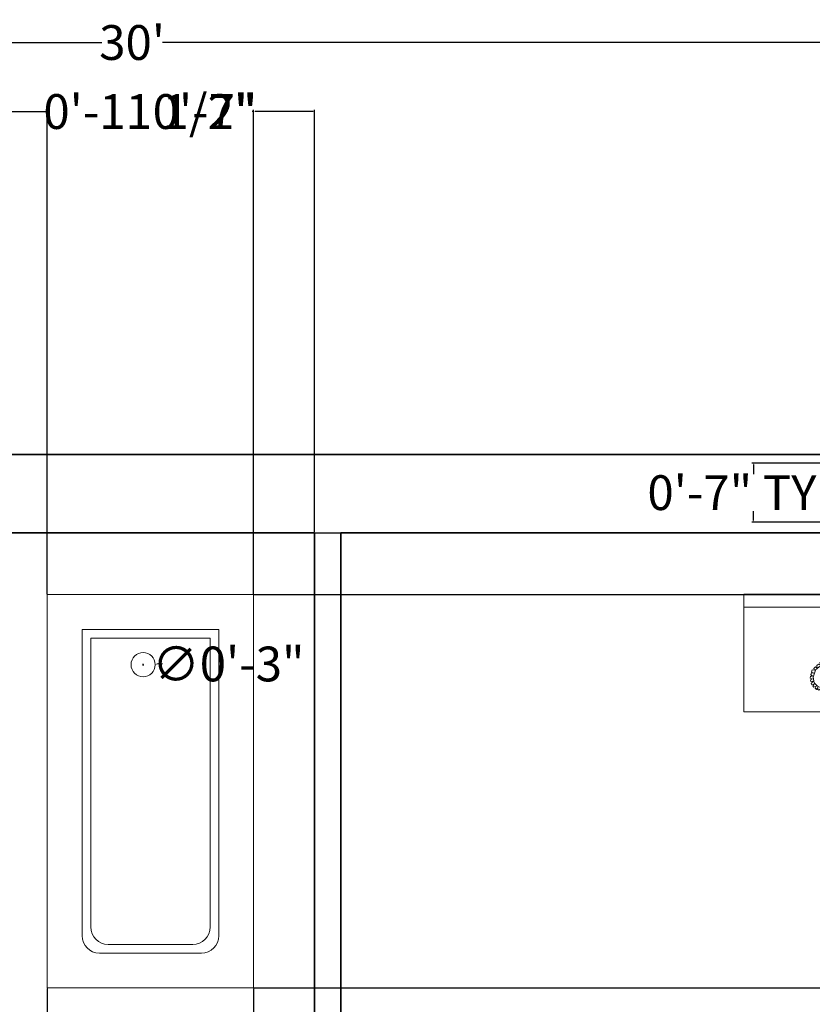
# Model space of a CAD drawing. Units: inches. Extents: x 311 to 754, y 60 to 497.
# Tile 10 of 11: x 530 to 621, y 384 to 497. Entities that reach past the tile are written whole.
import ezdxf

# ---------------------------------------------------------------- set-up
doc = ezdxf.new("R2010")
doc.units = ezdxf.units.IN
doc.header["$MEASUREMENT"] = 0
for name, color, linetype, lineweight in [('A-ANNO-DIMS', 2, 'Continuous', 18), ('A-FLOR-FIXT', 9, 'Continuous', 18), ('A-WALL', 7, 'Continuous', 35), ('beds', 70, 'Continuous', 13)]:
    doc.layers.add(name, color=color, linetype=linetype, lineweight=lineweight)
doc.styles.get("Standard").update_dxf_attribs({"font": 'arial.ttf'})
doc.dimstyles.get("Standard").update_dxf_attribs({"dimtxt": 4, "dimasz": 0.18, "dimexe": 0.18, "dimexo": 0.0625, "dimgap": 0.09, "dimtad": 0, "dimtih": 1, "dimtoh": 1, "dimdec": 0, "dimrnd": 6, "dimzin": 0, "dimdsep": 46, "dimlunit": 3, "dimtxsty": 'Standard', "dimcen": 0.09, "dimadec": 0, "dimazin": 0, "dimtfac": 1, "dimtdec": 0, "dimtofl": 0, "dimtmove": 0, "dimatfit": 3, "dimfxl": 1, "dimtolj": 1, "dimtzin": 0, "dimarcsym": 0})

# ---------------------------------------------------------------- blocks, each defined once
blk = doc.blocks.new('A$C57792D97')
for p, q in [((0.6, 2.6235), (0, 2.6235)), ((0, 2.6235), (0, 2.1735)), ((2.1, 2.6235), (0.6, 2.6235)), ((0.6, 2.6235), (0.6, 0.6235)), ((0.6, 0.6235), (0.6, 2.6235)), ((0.6, 2.1735), (0.6, 2.6235)), ((2.1, 0.6235), (2.1, 2.6235)), ((2.7, 2.6235), (2.1, 2.6235)), ((2.1, 2.6235), (2.1, 2.1735)), ((2.7, 2.1735), (2.7, 2.6235)), ((0.6, 2.5735), (0, 2.5735)), ((2.1, 2.5735), (0.6, 2.5735)), ((2.7, 2.5735), (2.1, 2.5735)), ((2.4103, 2.2312), (2.4103, 2.5317)), ((2.2593, 2.3802), (2.5698, 2.3802)), ((1.5491, 2.1955), (1.5516, 2.1955)), ((0, 2.1735), (0.6, 2.1735)), ((0.6, 2.1518), (0.8661, 2.1518)), ((2.1, 2.1735), (2.7, 2.1735)), ((0.6, 1.9518), (1.4767, 1.9518)), ((0.63, 0.6535), (0.63, 1.9518)), ((0.9906, 1.8942), (0.9508, 1.934)), ((1.4149, 1.8942), (1.3751, 1.934)), ((0.9906, 1.8942), (0.9344, 1.8942)), ((0.9906, 1.8942), (0.9508, 1.8544)), ((1.4149, 1.8942), (1.3586, 1.8942)), ((1.4149, 1.8942), (1.3751, 1.8544)), ((2.142, 1.8959), (2.1018, 1.8254)), ((2.1679, 1.8652), (2.1088, 1.8077)), ((2.1584, 1.8544), (2.1201, 1.8188)), ((2.1812, 1.8524), (2.1207, 1.8046)), ((2.1749, 1.8475), (2.1394, 1.7993)), ((2.1799, 1.8155), (2.1465, 1.7971)), ((2.2066, 1.8191), (2.1664, 1.7827)), ((2.249, 1.8154), (2.1711, 1.7709)), ((2.2173, 1.8274), (2.1931, 1.7688)), ((2.2496, 1.8292), (2.2008, 1.7642)), ((2.07, 1.7793), (2.07, 0.6535)), ((2.2713, 1.7954), (2.2055, 1.7458)), ((2.283, 1.7811), (2.2169, 1.7413)), ((2.2607, 1.7859), (2.2181, 1.7554)), ((2.2761, 1.777), (2.2348, 1.7337)), ((2.277, 1.7446), (2.2416, 1.7306)), ((2.304, 1.7449), (2.2596, 1.7138)), ((2.3456, 1.7359), (2.2627, 1.7015)), ((2.3157, 1.7518), (2.2843, 1.6966)), ((2.3479, 1.7495), (2.2914, 1.6911)), ((0.7785, 1.6821), (0.7387, 1.7219)), ((1.2027, 1.6821), (1.163, 1.7219)), ((1.627, 1.6821), (1.5872, 1.7219)), ((2.0513, 1.6821), (2.0115, 1.7219)), ((2.3653, 1.7133), (2.2937, 1.6723)), ((2.3751, 1.6976), (2.3045, 1.6664)), ((2.3535, 1.7051), (2.3075, 1.6802)), ((0.7785, 1.6821), (0.7222, 1.6821)), ((0.7785, 1.6821), (0.7387, 1.6423)), ((1.2027, 1.6821), (1.1465, 1.6821)), ((1.2027, 1.6821), (1.163, 1.6423)), ((1.627, 1.6821), (1.5708, 1.6821)), ((1.627, 1.6821), (1.5872, 1.6423)), ((2.0513, 1.6821), (1.995, 1.6821)), ((2.0513, 1.6821), (2.0115, 1.6423)), ((2.3677, 1.6944), (2.3213, 1.6565)), ((2.3645, 1.6621), (2.3277, 1.6526)), ((2.3913, 1.659), (2.3434, 1.6337)), ((2.4038, 1.6644), (2.3657, 1.6136)), ((2.4355, 1.6581), (2.372, 1.6073)), ((2.4314, 1.6449), (2.3449, 1.6211)), ((2.4482, 1.62), (2.372, 1.5882)), ((2.2754, 1.598), (2.2534, 1.5939)), ((2.2736, 1.5771), (2.2535, 1.594)), ((2.2736, 1.5771), (2.2754, 1.598)), ((2.4559, 1.6032), (2.382, 1.581)), ((2.4354, 1.6134), (2.3867, 1.5944)), ((2.4482, 1.6009), (2.3974, 1.5692)), ((2.3123, 1.541), (2.2911, 1.5481)), ((2.3006, 1.5236), (2.2912, 1.5481)), ((2.441, 1.5693), (2.4032, 1.5645)), ((2.4672, 1.5629), (2.4164, 1.5438)), ((2.4802, 1.5667), (2.4361, 1.5211)), ((2.5109, 1.5564), (2.4416, 1.514)), ((0.9906, 1.47), (0.9508, 1.5097)), ((1.4149, 1.47), (1.3751, 1.5097)), ((1.8391, 1.47), (1.7994, 1.5097)), ((2.3006, 1.5236), (2.3123, 1.541)), ((2.5052, 1.5438), (2.4164, 1.5311)), ((2.5187, 1.517), (2.4392, 1.4951)), ((2.5052, 1.5121), (2.4545, 1.4994)), ((0.9906, 1.47), (0.9344, 1.47)), ((0.9906, 1.47), (0.9508, 1.4302)), ((1.4149, 1.47), (1.3586, 1.47)), ((1.4149, 1.47), (1.3751, 1.4302)), ((1.8391, 1.47), (1.7829, 1.47)), ((1.8391, 1.47), (1.7994, 1.4302)), ((2.5243, 1.4994), (2.4482, 1.4867)), ((2.5163, 1.4981), (2.462, 1.473)), ((2.5052, 1.4677), (2.4672, 1.4677)), ((2.5658, 1.4343), (2.4761, 1.4328)), ((2.5304, 1.458), (2.4777, 1.4454)), ((2.5438, 1.4601), (2.4943, 1.4204)), ((2.573, 1.4461), (2.4989, 1.4127)), ((2.5758, 1.406), (2.4942, 1.3942)), ((2.5618, 1.4028), (2.5099, 1.3966)), ((2.5791, 1.3878), (2.502, 1.3848)), ((2.571, 1.3876), (2.514, 1.3695)), ((2.5562, 1.3587), (2.5185, 1.3635)), ((2.1596, 1.3147), (2.1502, 1.3392)), ((2.1714, 1.3321), (2.1502, 1.3392)), ((2.1596, 1.3147), (2.1714, 1.3321)), ((2.2534, 1.3469), (2.2315, 1.3429)), ((2.2516, 1.326), (2.2315, 1.3429)), ((2.2516, 1.326), (2.2535, 1.347)), ((2.3632, 1.3229), (2.33, 1.319)), ((2.3584, 1.2918), (2.33, 1.319)), ((2.3584, 1.2918), (2.3632, 1.3229)), ((2.6121, 1.3181), (2.523, 1.3279)), ((2.58, 1.346), (2.5261, 1.3402)), ((2.5936, 1.3464), (2.5395, 1.3132)), ((2.6207, 1.3289), (2.5431, 1.305)), ((0.7785, 1.2578), (0.7387, 1.2976)), ((1.2027, 1.2578), (1.163, 1.2976)), ((1.627, 1.2578), (1.5872, 1.2976)), ((2.0513, 1.2578), (2.0115, 1.2976)), ((2.6185, 1.2888), (2.5361, 1.2873)), ((2.6042, 1.2873), (2.5519, 1.2877)), ((0.7785, 1.2578), (0.7222, 1.2578)), ((0.7785, 1.2578), (0.7387, 1.218)), ((1.2027, 1.2578), (1.1465, 1.2578)), ((1.2027, 1.2578), (1.163, 1.218)), ((1.627, 1.2578), (1.5708, 1.2578)), ((1.627, 1.2578), (1.5872, 1.218)), ((2.0513, 1.2578), (1.995, 1.2578)), ((2.0513, 1.2578), (2.0115, 1.218)), ((2.4134, 1.2295), (2.404, 1.254)), ((2.4252, 1.2469), (2.404, 1.254)), ((2.4134, 1.2295), (2.4252, 1.2469)), ((2.6195, 1.2703), (2.5426, 1.277)), ((2.6115, 1.2711), (2.5526, 1.2603)), ((2.5932, 1.2443), (2.5563, 1.2538)), ((2.6435, 1.197), (2.5563, 1.2178)), ((2.6152, 1.2287), (2.561, 1.2296)), ((2.6287, 1.2274), (2.5709, 1.2013)), ((2.6534, 1.2066), (2.5734, 1.1926)), ((2.6462, 1.1671), (2.5642, 1.176)), ((2.6319, 1.1675), (2.58, 1.1743)), ((2.4947, 1.1445), (2.4728, 1.1404)), ((2.4929, 1.1236), (2.4728, 1.1404)), ((2.4929, 1.1236), (2.4948, 1.1445)), ((2.6449, 1.1486), (2.5694, 1.1649)), ((2.637, 1.1504), (2.5773, 1.147)), ((2.6155, 1.1261), (2.5801, 1.1402)), ((2.2315, 1.0959), (2.2095, 1.0919)), ((2.2297, 1.075), (2.2315, 1.0959)), ((2.6595, 1.0729), (2.5756, 1.1045)), ((2.6353, 1.1079), (2.5817, 1.1156)), ((2.6486, 1.1049), (2.588, 1.0862)), ((0.9906, 1.0457), (0.9508, 1.0855)), ((1.4149, 1.0457), (1.3751, 1.0855)), ((1.8391, 1.0457), (1.7994, 1.0855)), ((2.2297, 1.075), (2.2096, 1.0919)), ((2.6584, 1.0429), (2.5782, 1.062)), ((2.6705, 1.0812), (2.5894, 1.0774)), ((2.6442, 1.045), (2.5937, 1.0584)), ((0.9906, 1.0457), (0.9344, 1.0457)), ((0.9906, 1.0457), (0.9508, 1.0059)), ((1.4149, 1.0457), (1.3586, 1.0457)), ((1.4149, 1.0457), (1.3751, 1.0059)), ((1.8391, 1.0457), (1.7829, 1.0457)), ((1.8391, 1.0457), (1.7994, 1.0059)), ((2.2725, 1.0206), (2.2631, 1.0451)), ((2.2842, 1.038), (2.2631, 1.0451)), ((2.2725, 1.0206), (2.2843, 1.038)), ((2.6548, 1.0248), (2.582, 1.0503)), ((2.6472, 1.0275), (2.5875, 1.0316)), ((2.6228, 1.0061), (2.5895, 1.0244)), ((2.6598, 0.9477), (2.5805, 0.9897)), ((2.6402, 0.9855), (2.588, 0.9999)), ((2.653, 0.9809), (2.5905, 0.97)), ((2.3053, 0.9493), (2.272, 0.9455)), ((2.3005, 0.9182), (2.2721, 0.9455)), ((2.3005, 0.9182), (2.3053, 0.9494)), ((2.5263, 0.9355), (2.5169, 0.96)), ((2.538, 0.9528), (2.5169, 0.9599)), ((2.5263, 0.9355), (2.5381, 0.9529)), ((2.655, 0.9181), (2.5778, 0.9471)), ((2.6718, 0.9546), (2.5908, 0.961)), ((2.6412, 0.9221), (2.5927, 0.9416)), ((2.6491, 0.9006), (2.5801, 0.9351)), ((2.6419, 0.9043), (2.5832, 0.9159)), ((2.6151, 0.8861), (2.5843, 0.9085)), ((0.7785, 0.8336), (0.7387, 0.8733)), ((1.2027, 0.8336), (1.163, 0.8733)), ((1.627, 0.8336), (1.5872, 0.8733)), ((2.0513, 0.8336), (2.0115, 0.8733)), ((2.4728, 0.8934), (2.4508, 0.8894)), ((2.471, 0.8725), (2.4509, 0.8894)), ((2.471, 0.8725), (2.4728, 0.8934)), ((2.6444, 0.8236), (2.571, 0.8751)), ((2.6297, 0.8635), (2.5797, 0.8843)), ((0.7785, 0.8336), (0.7222, 0.8336)), ((0.7785, 0.8336), (0.7387, 0.7938)), ((1.2027, 0.8336), (1.1465, 0.8336)), ((1.2027, 0.8336), (1.163, 0.7938)), ((1.627, 0.8336), (1.5708, 0.8336)), ((1.627, 0.8336), (1.5872, 0.7938)), ((2.0513, 0.8336), (1.995, 0.8336)), ((2.0513, 0.8336), (2.0115, 0.7938)), ((2.1316, 0.8117), (2.1222, 0.8362)), ((2.1433, 0.8291), (2.1222, 0.8362)), ((2.1316, 0.8117), (2.1434, 0.8291)), ((2.2095, 0.8449), (2.1876, 0.8408)), ((2.2077, 0.824), (2.1876, 0.8408)), ((2.2077, 0.824), (2.2095, 0.8449)), ((2.6359, 0.7948), (2.5629, 0.8332)), ((2.6572, 0.8289), (2.5776, 0.8454)), ((2.6418, 0.8573), (2.5785, 0.8543)), ((1.9462, 0.7963), (1.9243, 0.7923)), ((2.6279, 0.7781), (2.5637, 0.821)), ((2.6212, 0.7827), (2.5644, 0.8015)), ((2.5923, 0.768), (2.5646, 0.7941)), ((2.6227, 0.8004), (2.577, 0.8259)), ((2.6136, 0.7023), (2.5472, 0.7626)), ((2.604, 0.7437), (2.557, 0.7707)), ((1.683, 0.7477), (1.661, 0.7437)), ((2.3854, 0.7265), (2.376, 0.751)), ((2.3971, 0.7439), (2.376, 0.751)), ((2.3854, 0.7265), (2.3972, 0.7439)), ((2.6016, 0.6748), (2.534, 0.7221)), ((2.6269, 0.706), (2.5501, 0.7323)), ((2.6153, 0.7361), (2.552, 0.7411)), ((1.4197, 0.6992), (1.3978, 0.6951)), ((2.5549, 0.6537), (2.5307, 0.6831)), ((2.5855, 0.6646), (2.5315, 0.6905)), ((2.5915, 0.6593), (2.5332, 0.7099)), ((2.5892, 0.6821), (2.547, 0.7131)), ((0.9906, 0.6214), (0.9508, 0.6612)), ((1.1564, 0.6506), (1.1345, 0.6466)), ((1.4149, 0.6214), (1.3751, 0.6612)), ((1.8391, 0.6214), (1.7994, 0.6612)), ((2.4508, 0.6424), (2.4289, 0.6383)), ((2.449, 0.6215), (2.4508, 0.6424)), ((2.5678, 0.5858), (2.5095, 0.654)), ((2.5635, 0.6282), (2.5203, 0.6608)), ((2.02, 0.6035), (0.6716, 0.6035)), ((0.9906, 0.6214), (0.9344, 0.6214)), ((0.9906, 0.6214), (0.9727, 0.6035)), ((1.4149, 0.6214), (1.3586, 0.6214)), ((1.4149, 0.6214), (1.397, 0.6035)), ((1.8391, 0.6214), (1.7829, 0.6214)), ((1.8391, 0.6214), (1.8212, 0.6035)), ((2.449, 0.6215), (2.4289, 0.6384)), ((2.5405, 0.546), (2.489, 0.6034)), ((2.5524, 0.5601), (2.4913, 0.6155)), ((2.541, 0.5688), (2.5031, 0.6049)), ((2.5815, 0.5878), (2.5085, 0.6236)), ((2.5737, 0.6192), (2.5116, 0.632)), ((0.6417, 0.5735), (2.05, 0.5735)), ((0.8932, 0.6021), (0.8712, 0.598)), ((1.3422, 0.5642), (1.3386, 0.5735)), ((1.3422, 0.5642), (1.3485, 0.5735)), ((2.1875, 0.5938), (2.1656, 0.5898)), ((2.1857, 0.5729), (2.1656, 0.5898)), ((2.1857, 0.5729), (2.1876, 0.5938)), ((2.2473, 0.5758), (2.2141, 0.5719)), ((2.2425, 0.5447), (2.2141, 0.572)), ((2.2425, 0.5447), (2.2474, 0.5758)), ((2.5035, 0.545), (2.4831, 0.5772)), ((2.5352, 0.552), (2.4849, 0.5844)), ((0.8062, 0.5164), (0.8823, 0.5291)), ((0.8142, 0.5177), (0.8685, 0.5428)), ((1.8485, 0.5294), (1.8152, 0.5255)), ((1.8437, 0.4983), (1.8485, 0.5294)), ((1.9243, 0.5453), (1.9023, 0.5412)), ((1.9225, 0.5244), (1.9024, 0.5412)), ((1.9225, 0.5244), (1.9243, 0.5453)), ((2.2445, 0.5176), (2.2351, 0.5421)), ((2.2445, 0.5176), (2.2562, 0.535)), ((2.5178, 0.5084), (2.4578, 0.5289)), ((2.5078, 0.476), (2.4585, 0.551)), ((2.5088, 0.5186), (2.47, 0.5564)), ((0.8118, 0.4988), (0.8913, 0.5207)), ((0.8196, 0.4594), (0.8889, 0.5018)), ((0.8253, 0.5037), (0.876, 0.5164)), ((0.8503, 0.4491), (0.8944, 0.4947)), ((1.6077, 0.4964), (1.5865, 0.5035)), ((1.596, 0.479), (1.5866, 0.5035)), ((1.596, 0.479), (1.6077, 0.4964)), ((1.661, 0.4967), (1.6391, 0.4927)), ((1.6592, 0.4758), (1.6391, 0.4927)), ((1.6592, 0.4758), (1.661, 0.4967)), ((1.8437, 0.4983), (1.8153, 0.5256)), ((2.4757, 0.4399), (2.4318, 0.5034)), ((2.4893, 0.4525), (2.4356, 0.515)), ((2.4791, 0.4625), (2.446, 0.503)), ((2.5216, 0.4763), (2.4537, 0.5209)), ((0.8253, 0.472), (0.9141, 0.4847)), ((0.8633, 0.4529), (0.9141, 0.472)), ((0.9592, 0.4578), (0.938, 0.4649)), ((0.9403, 0.459), (0.9381, 0.4649)), ((0.9508, 0.4454), (0.9592, 0.4578)), ((1.4496, 0.483), (1.4163, 0.4791)), ((1.4448, 0.4519), (1.4164, 0.4792)), ((1.4448, 0.4519), (1.4496, 0.483)), ((2.4345, 0.3746), (2.395, 0.4552)), ((2.4409, 0.4167), (2.4071, 0.4591)), ((2.4389, 0.4436), (2.4227, 0.478)), ((2.4712, 0.4466), (2.4253, 0.485)), ((0.8746, 0.4126), (0.9485, 0.4347)), ((0.8823, 0.4149), (0.9331, 0.4466)), ((0.8823, 0.3958), (0.9585, 0.4275)), ((0.8895, 0.4465), (0.9273, 0.4513)), ((0.8951, 0.4024), (0.9438, 0.4214)), ((1.0507, 0.4366), (1.0175, 0.4327)), ((1.0459, 0.4055), (1.0175, 0.4328)), ((1.0459, 0.4055), (1.0507, 0.4366)), ((1.3977, 0.4481), (1.3758, 0.4441)), ((1.3959, 0.4272), (1.3758, 0.4441)), ((1.3959, 0.4272), (1.3978, 0.4482)), ((1.8615, 0.4113), (1.8403, 0.4184)), ((1.8498, 0.3939), (1.8404, 0.4184)), ((2.4132, 0.3535), (2.3678, 0.4224)), ((2.4482, 0.3731), (2.3865, 0.4259)), ((2.4485, 0.4055), (2.3915, 0.4334)), ((0.895, 0.3577), (0.9585, 0.4085)), ((0.8991, 0.3709), (0.9856, 0.3946)), ((0.9267, 0.3514), (0.9648, 0.4022)), ((0.9392, 0.3568), (0.9872, 0.3821)), ((1.1345, 0.3996), (1.1125, 0.3955)), ((1.1327, 0.3787), (1.1126, 0.3955)), ((1.1327, 0.3787), (1.1345, 0.3996)), ((1.213, 0.3727), (1.1918, 0.3798)), ((1.2013, 0.3553), (1.1919, 0.3798)), ((1.8498, 0.3939), (1.8615, 0.4113)), ((2.3621, 0.3511), (2.3503, 0.3873)), ((2.3945, 0.35), (2.3538, 0.3939)), ((2.3981, 0.3428), (2.3625, 0.4113)), ((2.4043, 0.3648), (2.3766, 0.4092)), ((0.9555, 0.3182), (1.026, 0.3494)), ((0.9628, 0.3214), (1.0092, 0.3592)), ((0.9652, 0.3025), (1.0368, 0.3435)), ((0.966, 0.3537), (1.0029, 0.3631)), ((1.2013, 0.3553), (1.213, 0.3727)), ((2.1656, 0.3428), (2.1436, 0.3387)), ((2.1638, 0.3219), (2.1656, 0.3428)), ((2.3625, 0.28), (2.3078, 0.3401)), ((2.3668, 0.3121), (2.3138, 0.3469)), ((2.3491, 0.2832), (2.32, 0.3681)), ((2.3607, 0.3242), (2.3324, 0.3704)), ((0.977, 0.3107), (1.023, 0.3356)), ((0.9826, 0.2663), (1.0392, 0.3246)), ((0.9849, 0.2799), (1.0678, 0.3143)), ((1.0148, 0.264), (1.0462, 0.3191)), ((1.0265, 0.2709), (1.0709, 0.302)), ((2.1153, 0.3261), (2.0941, 0.3332)), ((2.1036, 0.3087), (2.0942, 0.3332)), ((2.1036, 0.3087), (2.1153, 0.3261)), ((2.1638, 0.3219), (2.1437, 0.3388)), ((2.2743, 0.2689), (2.2671, 0.3063)), ((2.3063, 0.2638), (2.2714, 0.3124)), ((2.309, 0.2562), (2.2823, 0.3286)), ((2.3253, 0.265), (2.2888, 0.3389)), ((2.3179, 0.2773), (2.2959, 0.3247)), ((1.0475, 0.2347), (1.1136, 0.2745)), ((1.0535, 0.2712), (1.0889, 0.2852)), ((1.0544, 0.2388), (1.0957, 0.2821)), ((1.0592, 0.2203), (1.125, 0.27)), ((1.4668, 0.2875), (1.4456, 0.2946)), ((1.4551, 0.2701), (1.4457, 0.2946)), ((1.4551, 0.2701), (1.4668, 0.2875)), ((1.9023, 0.2942), (1.8804, 0.2902)), ((1.9005, 0.2733), (1.8804, 0.2902)), ((1.9005, 0.2733), (1.9023, 0.2942)), ((2.227, 0.1881), (2.2001, 0.2661)), ((2.2658, 0.1984), (2.2191, 0.2649)), ((2.2741, 0.2296), (2.2258, 0.2708)), ((2.2529, 0.2032), (2.2346, 0.291)), ((2.2695, 0.2424), (2.2473, 0.2918)), ((1.0699, 0.2299), (1.1124, 0.2604)), ((1.0809, 0.1866), (1.1297, 0.2516)), ((1.0815, 0.2004), (1.1594, 0.2449)), ((1.1132, 0.1884), (1.1374, 0.247)), ((1.1239, 0.1967), (1.1641, 0.2331)), ((1.639, 0.2457), (1.6171, 0.2416)), ((1.6372, 0.2248), (1.6171, 0.2416)), ((1.6372, 0.2248), (1.6391, 0.2457)), ((2.1768, 0.1984), (2.1745, 0.2364)), ((2.208, 0.1893), (2.1795, 0.2419)), ((2.2097, 0.1814), (2.1923, 0.2566)), ((2.2212, 0.2012), (2.2053, 0.2511)), ((1.1493, 0.1634), (1.2098, 0.2112)), ((1.1507, 0.2003), (1.184, 0.2187)), ((1.1556, 0.1683), (1.1911, 0.2165)), ((1.1626, 0.1506), (1.2217, 0.2081)), ((1.1721, 0.1614), (1.2104, 0.197)), ((1.1885, 0.1199), (1.2287, 0.1904)), ((1.3758, 0.1971), (1.3538, 0.193)), ((1.374, 0.1762), (1.3539, 0.1931)), ((1.374, 0.1762), (1.3758, 0.1971)), ((1.7206, 0.2023), (1.6994, 0.2094)), ((1.7089, 0.1849), (1.6995, 0.2095)), ((1.7089, 0.1849), (1.7206, 0.2024)), ((2.1018, 0.1197), (2.0939, 0.1965)), ((2.1198, 0.1242), (2.1029, 0.2049)), ((2.1157, 0.1379), (2.1062, 0.1893)), ((2.1596, 0.1295), (2.1216, 0.2013)), ((2.1718, 0.1594), (2.129, 0.2063)), ((2.1474, 0.1359), (2.1403, 0.2253)), ((2.1688, 0.1727), (2.1529, 0.2245)), ((1.1873, 0.1336), (1.259, 0.1875)), ((1.2203, 0.1256), (1.237, 0.1868)), ((1.2299, 0.1352), (1.2652, 0.1764)), ((1.2559, 0.1422), (1.2867, 0.1646)), ((1.2592, 0.1054), (1.3133, 0.1604)), ((1.2649, 0.111), (1.2941, 0.1633)), ((1.2741, 0.0944), (1.3255, 0.1588)), ((1.7905, 0.1559), (1.7573, 0.152)), ((1.7857, 0.1248), (1.7573, 0.152)), ((1.7857, 0.1248), (1.7906, 0.1559)), ((2.0054, 0.0742), (1.9988, 0.1564)), ((2.0614, 0.1027), (2.0249, 0.1545)), ((2.0343, 0.0824), (2.0385, 0.172)), ((2.0601, 0.1162), (2.0509, 0.1696)), ((2.0714, 0.1407), (2.0737, 0.1787)), ((2.1011, 0.1277), (2.0794, 0.1835)), ((1.282, 0.1063), (1.3156, 0.1464)), ((1.3007, 0.0806), (1.3651, 0.1431)), ((1.3035, 0.0671), (1.3346, 0.1421)), ((1.3344, 0.0768), (1.3433, 0.1396)), ((1.3427, 0.0876), (1.3725, 0.1328)), ((1.3677, 0.0977), (1.3954, 0.1238)), ((1.3755, 0.0616), (1.4223, 0.1229)), ((1.3804, 0.0679), (1.4028, 0.1234)), ((1.3916, 0.0525), (1.4346, 0.1229)), ((1.8672, 0.039), (1.8787, 0.1154)), ((1.8857, 0.0389), (1.8894, 0.1213)), ((1.9256, 0.0342), (1.9067, 0.1132)), ((1.9448, 0.0601), (1.9151, 0.1162)), ((1.9154, 0.0434), (1.9307, 0.1318)), ((1.9452, 0.0737), (1.9428, 0.1279)), ((1.9595, 0.0966), (1.9666, 0.134)), ((1.9873, 0.08), (1.9728, 0.1381)), ((1.9871, 0.072), (1.9889, 0.1491)), ((2.0031, 0.0883), (2.0001, 0.1405)), ((2.0456, 0.0745), (2.0169, 0.1505)), ((1.3981, 0.0653), (1.4264, 0.1093)), ((1.4198, 0.0422), (1.4758, 0.1123)), ((1.4243, 0.0292), (1.4458, 0.1075)), ((1.4537, 0.0427), (1.4546, 0.1061)), ((1.4606, 0.0544), (1.4845, 0.103)), ((1.4841, 0.0676), (1.5083, 0.0969)), ((1.4964, 0.0327), (1.5351, 0.0995)), ((1.5005, 0.0397), (1.5158, 0.0975)), ((1.5135, 0.0258), (1.5473, 0.101)), ((1.5183, 0.0393), (1.5409, 0.0865)), ((1.5428, 0.0191), (1.5896, 0.0956)), ((1.5489, 0.0067), (1.5603, 0.0871)), ((1.5763, 0.0238), (1.5693, 0.0868)), ((1.5817, 0.0362), (1.5994, 0.0875)), ((1.6034, 0.0523), (1.6237, 0.0845)), ((1.6199, 0.0192), (1.65, 0.0903)), ((1.6232, 0.0266), (1.631, 0.086)), ((1.6378, 0.0145), (1.6619, 0.0934)), ((1.6409, 0.0285), (1.6573, 0.0782)), ((1.6677, 0.0115), (1.7045, 0.0933)), ((1.6753, 0), (1.6766, 0.0812)), ((1.7004, 0.0204), (1.6855, 0.0821)), ((1.7041, 0.0334), (1.7152, 0.0865)), ((1.7236, 0.0521), (1.7398, 0.0865)), ((1.7442, 0.0214), (1.7651, 0.0956)), ((1.7465, 0.0291), (1.7469, 0.0889)), ((1.7625, 0.0189), (1.7765, 0.1002)), ((1.7638, 0.0332), (1.7739, 0.0845)), ((1.7925, 0.0197), (1.8188, 0.1054)), ((1.8015, 0.0092), (1.7926, 0.09)), ((1.8238, 0.0326), (1.8014, 0.0919)), ((1.8259, 0.046), (1.8303, 0.1)), ((1.8429, 0.0669), (1.8547, 0.1031)), ((1.8685, 0.047), (1.8614, 0.1064)), ((1.8852, 0.0532), (1.8888, 0.1054))]:
    blk.add_line(p, q)
at = {"linetype": 'ByBlock'}
for p, q in [((0.3217, 2.5511), (0.3189, 2.5483)), ((0.3189, 2.5483), (0.3189, 2.3511)), ((0.5475, 2.5511), (0.3217, 2.5511)), ((0.3375, 2.5469), (0.3303, 2.5397)), ((0.3303, 2.5397), (0.3303, 2.3683)), ((0.3346, 2.5426), (0.3332, 2.5369)), ((0.3332, 2.5369), (0.3332, 2.4983)), ((0.3332, 2.5369), (0.346, 2.524)), ((0.3403, 2.5454), (0.3346, 2.5426)), ((0.3803, 2.5469), (0.3375, 2.5469)), ((0.3746, 2.5454), (0.3403, 2.5454)), ((0.3475, 2.5269), (0.3403, 2.5454)), ((0.346, 2.524), (0.3475, 2.5269)), ((0.346, 2.4597), (0.346, 2.524)), ((0.3475, 2.5269), (0.3675, 2.5269)), ((0.3675, 2.5269), (0.3746, 2.5454)), ((0.3689, 2.524), (0.3675, 2.5269)), ((0.3818, 2.5369), (0.3689, 2.524)), ((0.3689, 2.4597), (0.3689, 2.524)), ((0.3746, 2.5454), (0.3803, 2.5426)), ((0.386, 2.5397), (0.3803, 2.5469)), ((0.3803, 2.5426), (0.3818, 2.5369)), ((0.3818, 2.5369), (0.3818, 2.4983)), ((0.386, 2.3668), (0.386, 2.5397)), ((0.3989, 2.4597), (0.3989, 2.5354)), ((0.3989, 2.5354), (0.5418, 2.5354)), ((0.5418, 2.5354), (0.5418, 2.4597)), ((0.5475, 2.5511), (0.5503, 2.5483)), ((0.5503, 2.5483), (0.5503, 2.3511)), ((0.3332, 2.4983), (0.336, 2.4911)), ((0.336, 2.4911), (0.3403, 2.484)), ((0.3789, 2.4911), (0.3746, 2.484)), ((0.3818, 2.4983), (0.3789, 2.4911)), ((0.3403, 2.484), (0.3417, 2.474)), ((0.3417, 2.474), (0.3417, 2.4597)), ((0.3417, 2.4326), (0.3417, 2.4597)), ((0.346, 2.4597), (0.346, 2.3826)), ((0.3689, 2.4597), (0.3689, 2.3826)), ((0.3746, 2.484), (0.3732, 2.474)), ((0.3732, 2.474), (0.3732, 2.4597)), ((0.3732, 2.4326), (0.3732, 2.4597)), ((0.5418, 2.4597), (0.3989, 2.4597)), ((0.3989, 2.4426), (0.3989, 2.4568)), ((0.3989, 2.4568), (0.5361, 2.4568)), ((0.4675, 2.4568), (0.4675, 2.4426)), ((0.4789, 2.4568), (0.4789, 2.4426)), ((0.4903, 2.4568), (0.4903, 2.4426)), ((0.5018, 2.4568), (0.5018, 2.4426)), ((0.5132, 2.4568), (0.5132, 2.4426)), ((0.5246, 2.4568), (0.5246, 2.4426)), ((0.5361, 2.4568), (0.5361, 2.4426)), ((0.3332, 2.4083), (0.336, 2.4154)), ((0.336, 2.4154), (0.3403, 2.4226)), ((0.3403, 2.4226), (0.3417, 2.4326)), ((0.3746, 2.4226), (0.3732, 2.4326)), ((0.3789, 2.4154), (0.3746, 2.4226)), ((0.3818, 2.4083), (0.3789, 2.4154)), ((0.5361, 2.4426), (0.3989, 2.4426)), ((0.3989, 2.4197), (0.3989, 2.4111)), ((0.4103, 2.4197), (0.3989, 2.4197)), ((0.3989, 2.4111), (0.4103, 2.4111)), ((0.4103, 2.4111), (0.4103, 2.4197)), ((0.4275, 2.4197), (0.416, 2.4197)), ((0.416, 2.4197), (0.416, 2.4111)), ((0.416, 2.4111), (0.4275, 2.4111)), ((0.4275, 2.4111), (0.4275, 2.4197)), ((0.4332, 2.4197), (0.4332, 2.4111)), ((0.4446, 2.4197), (0.4332, 2.4197)), ((0.4332, 2.4111), (0.4446, 2.4111)), ((0.4446, 2.4111), (0.4446, 2.4197)), ((0.4575, 2.4011), (0.4575, 2.4268)), ((0.4575, 2.4268), (0.5418, 2.4268)), ((0.4718, 2.424), (0.4761, 2.424)), ((0.4718, 2.4197), (0.4718, 2.424)), ((0.4761, 2.4197), (0.4718, 2.4197)), ((0.4761, 2.424), (0.4761, 2.4197)), ((0.4975, 2.424), (0.5018, 2.424)), ((0.4975, 2.4197), (0.4975, 2.424)), ((0.5018, 2.4197), (0.4975, 2.4197)), ((0.5018, 2.424), (0.5018, 2.4197)), ((0.5232, 2.4197), (0.5232, 2.424)), ((0.5232, 2.424), (0.5275, 2.424)), ((0.5275, 2.4197), (0.5232, 2.4197)), ((0.5275, 2.424), (0.5275, 2.4197)), ((0.5418, 2.4268), (0.5418, 2.4011)), ((0.3063, 2.3696), (0.3103, 2.3737)), ((0.3103, 2.3737), (0.3189, 2.3768)), ((0.3332, 2.3697), (0.3332, 2.4083)), ((0.3332, 2.3697), (0.346, 2.3826)), ((0.3475, 2.3797), (0.3403, 2.3611)), ((0.346, 2.3826), (0.3475, 2.3797)), ((0.3475, 2.3797), (0.3675, 2.3797)), ((0.3689, 2.3826), (0.3675, 2.3797)), ((0.3675, 2.3797), (0.3746, 2.3611)), ((0.3818, 2.3697), (0.3689, 2.3826)), ((0.3818, 2.3697), (0.3818, 2.4083)), ((0.3989, 2.404), (0.3989, 2.3954)), ((0.4103, 2.404), (0.3989, 2.404)), ((0.3989, 2.3954), (0.4103, 2.3954)), ((0.4103, 2.3883), (0.3989, 2.3883)), ((0.3989, 2.3883), (0.3989, 2.3797)), ((0.3989, 2.3797), (0.4103, 2.3797)), ((0.4103, 2.3954), (0.4103, 2.404)), ((0.4103, 2.3797), (0.4103, 2.3883)), ((0.416, 2.404), (0.416, 2.3954)), ((0.4275, 2.404), (0.416, 2.404)), ((0.416, 2.3954), (0.4275, 2.3954)), ((0.4275, 2.3868), (0.416, 2.3868)), ((0.416, 2.3868), (0.416, 2.3783)), ((0.416, 2.3783), (0.4275, 2.3783)), ((0.4275, 2.3954), (0.4275, 2.404)), ((0.4275, 2.3783), (0.4275, 2.3868)), ((0.4332, 2.404), (0.4332, 2.3954)), ((0.4446, 2.404), (0.4332, 2.404)), ((0.4332, 2.3954), (0.4446, 2.3954)), ((0.4446, 2.3868), (0.4332, 2.3868)), ((0.4332, 2.3868), (0.4332, 2.3783)), ((0.4332, 2.3783), (0.4446, 2.3783)), ((0.4446, 2.3954), (0.4446, 2.404)), ((0.4446, 2.3783), (0.4446, 2.3868)), ((0.5418, 2.4011), (0.4575, 2.4011)), ((0.4661, 2.394), (0.4803, 2.394)), ((0.4661, 2.3883), (0.4661, 2.394)), ((0.4803, 2.3883), (0.4661, 2.3883)), ((0.4718, 2.4083), (0.4761, 2.4083)), ((0.4718, 2.404), (0.4718, 2.4083)), ((0.4761, 2.404), (0.4718, 2.404)), ((0.4761, 2.4083), (0.4761, 2.404)), ((0.4803, 2.394), (0.4803, 2.3883)), ((0.4861, 2.3883), (0.4861, 2.394)), ((0.4861, 2.394), (0.5003, 2.394)), ((0.5003, 2.3883), (0.4861, 2.3883)), ((0.4975, 2.4083), (0.5018, 2.4083)), ((0.4975, 2.404), (0.4975, 2.4083)), ((0.5018, 2.404), (0.4975, 2.404)), ((0.5003, 2.394), (0.5003, 2.3883)), ((0.5018, 2.4083), (0.5018, 2.404)), ((0.5061, 2.3883), (0.5061, 2.394)), ((0.5061, 2.394), (0.5203, 2.394)), ((0.5203, 2.3883), (0.5061, 2.3883)), ((0.5203, 2.394), (0.5203, 2.3883)), ((0.5232, 2.4083), (0.5275, 2.4083)), ((0.5232, 2.404), (0.5232, 2.4083)), ((0.5275, 2.404), (0.5232, 2.404)), ((0.5261, 2.3883), (0.5261, 2.394)), ((0.5261, 2.394), (0.5403, 2.394)), ((0.5403, 2.3883), (0.5261, 2.3883)), ((0.5275, 2.4083), (0.5275, 2.404)), ((0.5403, 2.394), (0.5403, 2.3883)), ((0.2683, 2.3394), (0.2738, 2.3452)), ((0.2706, 2.3331), (0.2683, 2.3394)), ((0.2738, 2.3452), (0.2804, 2.3412)), ((0.2937, 2.3497), (0.2748, 2.3336)), ((0.2789, 2.3502), (0.2854, 2.3565)), ((0.2804, 2.3412), (0.2789, 2.3502)), ((0.2854, 2.3565), (0.2932, 2.3525)), ((0.2902, 2.3608), (0.294, 2.3648)), ((0.2932, 2.3525), (0.2902, 2.3608)), ((0.3053, 2.3601), (0.2937, 2.3497)), ((0.294, 2.3648), (0.2975, 2.3621)), ((0.2955, 2.3663), (0.298, 2.3689)), ((0.2975, 2.3621), (0.2955, 2.3663)), ((0.298, 2.3689), (0.3033, 2.3669)), ((0.3053, 2.3628), (0.3023, 2.3631)), ((0.3023, 2.3631), (0.3053, 2.3601)), ((0.3033, 2.3669), (0.3063, 2.3696)), ((0.3068, 2.3648), (0.3053, 2.3628)), ((0.3126, 2.3694), (0.3068, 2.3648)), ((0.3189, 2.3711), (0.3126, 2.3694)), ((0.3189, 2.3511), (0.3217, 2.3483)), ((0.3217, 2.3483), (0.3525, 2.3483)), ((0.3303, 2.3683), (0.3375, 2.3597)), ((0.3346, 2.364), (0.3332, 2.3697)), ((0.3403, 2.3611), (0.3346, 2.364)), ((0.3375, 2.3597), (0.3542, 2.3597)), ((0.3543, 2.3611), (0.3403, 2.3611)), ((0.3483, 2.3311), (0.3518, 2.3447)), ((0.3518, 2.3447), (0.3538, 2.354)), ((0.3552, 2.3386), (0.3518, 2.325)), ((0.3538, 2.354), (0.3546, 2.3654)), ((0.3546, 2.3654), (0.3589, 2.3654)), ((0.3587, 2.3531), (0.3552, 2.3386)), ((0.3575, 2.3483), (0.5475, 2.3483)), ((0.3589, 2.3654), (0.3587, 2.3531)), ((0.3746, 2.3611), (0.3588, 2.3611)), ((0.3588, 2.3597), (0.3789, 2.3597)), ((0.3746, 2.3611), (0.3803, 2.364)), ((0.3789, 2.3597), (0.386, 2.3668)), ((0.3803, 2.364), (0.3818, 2.3697)), ((0.4103, 2.3711), (0.3989, 2.3711)), ((0.3989, 2.3711), (0.3989, 2.3626)), ((0.3989, 2.3626), (0.4103, 2.3626)), ((0.4103, 2.3626), (0.4103, 2.3711)), ((0.416, 2.3711), (0.416, 2.3626)), ((0.4275, 2.3711), (0.416, 2.3711)), ((0.416, 2.3626), (0.4275, 2.3626)), ((0.4275, 2.3626), (0.4275, 2.3711)), ((0.4332, 2.3711), (0.4332, 2.3626)), ((0.4446, 2.3711), (0.4332, 2.3711)), ((0.4332, 2.3626), (0.4446, 2.3626)), ((0.4446, 2.3626), (0.4446, 2.3711)), ((0.4661, 2.3726), (0.4661, 2.364)), ((0.4803, 2.3726), (0.4661, 2.3726)), ((0.4661, 2.364), (0.4803, 2.364)), ((0.4803, 2.364), (0.4803, 2.3726)), ((0.5003, 2.3726), (0.4861, 2.3726)), ((0.4861, 2.3726), (0.4861, 2.364)), ((0.4861, 2.364), (0.5003, 2.364)), ((0.5003, 2.364), (0.5003, 2.3726)), ((0.5203, 2.3726), (0.5061, 2.3726)), ((0.5061, 2.3726), (0.5061, 2.364)), ((0.5061, 2.364), (0.5203, 2.364)), ((0.5203, 2.364), (0.5203, 2.3726)), ((0.5403, 2.3726), (0.5261, 2.3726)), ((0.5261, 2.3726), (0.5261, 2.364)), ((0.5261, 2.364), (0.5403, 2.364)), ((0.5403, 2.364), (0.5403, 2.3726)), ((0.5503, 2.3511), (0.5475, 2.3483)), ((0.2532, 2.3027), (0.2546, 2.31)), ((0.2621, 2.3001), (0.2532, 2.3027)), ((0.2546, 2.31), (0.2624, 2.31)), ((0.2546, 2.2958), (0.2621, 2.3001)), ((0.2563, 2.3158), (0.2584, 2.3224)), ((0.2624, 2.31), (0.2563, 2.3158)), ((0.2584, 2.3224), (0.2676, 2.3221)), ((0.2592, 2.3253), (0.2618, 2.334)), ((0.2676, 2.3221), (0.2592, 2.3253)), ((0.2618, 2.334), (0.2705, 2.3331)), ((0.2746, 2.3331), (0.265, 2.3059)), ((0.265, 2.3059), (0.2691, 2.2842)), ((0.3422, 2.288), (0.3437, 2.3062)), ((0.3425, 2.3129), (0.3477, 2.3166)), ((0.3437, 2.3062), (0.3425, 2.3129)), ((0.3549, 2.3056), (0.3466, 2.3042)), ((0.3466, 2.3042), (0.3546, 2.2993)), ((0.3474, 2.3242), (0.3483, 2.3311)), ((0.3477, 2.3166), (0.3474, 2.3242)), ((0.352, 2.3175), (0.3512, 2.3158)), ((0.3512, 2.3158), (0.3544, 2.3126)), ((0.3518, 2.325), (0.352, 2.3175)), ((0.3546, 2.2993), (0.3541, 2.2915)), ((0.3544, 2.3126), (0.3549, 2.3056)), ((0.2558, 2.29), (0.2546, 2.2958)), ((0.2647, 2.2903), (0.2558, 2.29)), ((0.2578, 2.2825), (0.2647, 2.2903)), ((0.2601, 2.2767), (0.2578, 2.2825)), ((0.2685, 2.2793), (0.2601, 2.2767)), ((0.2644, 2.2715), (0.2685, 2.2793)), ((0.2682, 2.268), (0.2644, 2.2715)), ((0.2763, 2.2715), (0.2682, 2.268)), ((0.2691, 2.2842), (0.2818, 2.2718)), ((0.2728, 2.2637), (0.2763, 2.2715)), ((0.2774, 2.2596), (0.2728, 2.2637)), ((0.2835, 2.2672), (0.2774, 2.2596)), ((0.2818, 2.2718), (0.2986, 2.2646)), ((0.2827, 2.2585), (0.2835, 2.2672)), ((0.2939, 2.262), (0.2873, 2.2562)), ((0.2942, 2.2541), (0.2939, 2.262)), ((0.2986, 2.2646), (0.3159, 2.266)), ((0.3029, 2.262), (0.2997, 2.2527)), ((0.3049, 2.2536), (0.3029, 2.262)), ((0.3133, 2.262), (0.3098, 2.2541)), ((0.3171, 2.2541), (0.3133, 2.262)), ((0.3159, 2.266), (0.3312, 2.2741)), ((0.3292, 2.2596), (0.3223, 2.2654)), ((0.3223, 2.2654), (0.3231, 2.2559)), ((0.3347, 2.2631), (0.3292, 2.2596)), ((0.3312, 2.2741), (0.3422, 2.288)), ((0.3402, 2.266), (0.3335, 2.2709)), ((0.3335, 2.2709), (0.3347, 2.2631)), ((0.3445, 2.2712), (0.3402, 2.266)), ((0.3492, 2.2776), (0.3405, 2.2793)), ((0.3405, 2.2793), (0.3445, 2.2712)), ((0.3541, 2.2915), (0.3448, 2.2906)), ((0.3448, 2.2906), (0.3529, 2.2842)), ((0.3529, 2.2842), (0.3492, 2.2776)), ((0.2873, 2.2562), (0.2827, 2.2585)), ((0.2997, 2.2527), (0.2942, 2.2541)), ((0.3098, 2.2541), (0.3049, 2.2536)), ((0.3231, 2.2559), (0.3171, 2.2541))]:
    blk.add_line(p, q, dxfattribs=at)
for centre, radius in [((2.4068, 2.3792), 0.1082), ((2.4128, 2.3792), 0.062)]:
    blk.add_circle(centre, radius)
for centre, radius, start, end in [((0.8117, 1.4495), 1.1155, 75.3755, 98.4519), ((1.5803, 0.4369), 2.1259, 84.0997, 95.547), ((0.7133, 2.123), 0.4349, 62.6153, 98.6623), ((0.9995, 2.5566), 0.3518, 180.6066, 203.849), ((1.2711, 1.6927), 0.8548, 85.0132, 101.9962), ((0.9942, 1.5092), 1.0245, 76.8495, 84.445), ((-2.6554, 2.4937), 4.0011, 355.9906, 0.7251), ((7.229, 2.8402), 5.8612, 182.80995, 184.16642), ((1.505, 1.754), 0.7941, 71.9705, 99.0452), ((2.0384, 6.4739), 3.9297, 266.5056, 270.1818), ((1.6997, 1.5092), 1.0245, 76.8495, 84.445), ((2.5231, 2.3654), 0.505, 159.2551, 197.4606), ((6.5168, 1.1676), 5.2262, 165.6998, 168.4122), ((1.7461, 2.3905), 1.0686, 178.7205, 189.3246), ((2.4516, 2.3905), 1.0686, 178.7205, 189.3246), ((1.0382, 2.187), 0.3479, 146.8128, 174.9884), ((1.3553, 2.3447), 0.1322, 217.4973, 261.5591), ((2.6076, 3.8927), 1.7717, 246.8027, 251.3608), ((0.9964, 4.7934), 2.5939, 263.2521, 270.4789), ((1.1218, 3.4256), 1.2305, 265.1643, 280.0187), ((1.5587, 3.1365), 0.9332, 260.0314, 280.1788), ((1.8907, 2.8521), 0.6558, 255.2386, 283.2855), ((1.0153, 0.392), 1.7661, 72.4208, 94.846), ((0.7898, 0.8867), 1.2674, 53.0057, 86.5496), ((2.0108, 3.233), 1.2462, 248.2311, 274.1028), ((1.991, 2.6169), 0.8413, 238.5747, 277.4412), ((1.6653, 1.0079), 0.9493, 207.2312, 62.7432), ((1.6653, 1.0079), 0.9093, 208.5361, 61.4369), ((0.6787, 0.6517), 0.0487, 177.8916, 261.664), ((2.02, 0.6535), 0.05, 270, 0), ((0.6518, 0.6244), 0.0518, 180.9151, 258.7324), ((2.05, 0.6235), 0.05, 270, 0)]:
    blk.add_arc(centre, radius, start, end)
blk = doc.blocks.new('*D103')
at = {"layer": 'A-ANNO-DIMS', "color": 0, "lineweight": -2, "transparency": 16777216}
for p, q in [((362.8, 447.3), (362.8, 494.8)), ((722.8, 447.3), (722.8, 494.8)), ((362.98, 494.62), (539.32, 494.62)), ((722.62, 494.62), (546.29, 494.62))]:
    blk.add_line(p, q, dxfattribs=at)
at = {"layer": 'A-ANNO-DIMS', "color": 0, "transparency": 16777216}
for points in [[(362.98, 494.65), (362.98, 494.59), (362.8, 494.62)], [(722.62, 494.65), (722.62, 494.59), (722.8, 494.62)]]:
    blk.add_solid(points, dxfattribs=at)
at = {"layer": 'Defpoints', "color": 0, "transparency": 16777216}
for p in [(722.8, 494.62), (362.8, 447.24), (722.8, 447.24)]:
    blk.add_point(p, dxfattribs=at)
at = {"layer": 'A-ANNO-DIMS', "color": 0, "transparency": 16777216, "insert": (542.8, 494.62), "char_height": 4, "attachment_point": 5}
blk.add_mtext("\\A1;30'", dxfattribs=at)
blk = doc.blocks.new('*D107')
at = {"layer": 'A-ANNO-DIMS', "color": 0, "lineweight": -2, "transparency": 16777216}
for p, q in [((623.07, 446.26), (614.12, 446.26)), ((614.3, 446.08), (614.3, 444.99)), ((614.3, 439.64), (614.3, 440.73)), ((623.07, 439.46), (614.12, 439.46))]:
    blk.add_line(p, q, dxfattribs=at)
at = {"layer": 'A-ANNO-DIMS', "color": 0, "transparency": 16777216}
for points in [[(614.27, 446.08), (614.33, 446.08), (614.3, 446.26)], [(614.27, 439.64), (614.33, 439.64), (614.3, 439.46)]]:
    blk.add_solid(points, dxfattribs=at)
at = {"layer": 'Defpoints', "color": 0, "transparency": 16777216}
for p in [(614.3, 446.26), (623.13, 446.26), (623.13, 439.46)]:
    blk.add_point(p, dxfattribs=at)
at = {"layer": 'A-ANNO-DIMS', "color": 0, "transparency": 16777216, "insert": (614.3, 442.86), "char_height": 4, "attachment_point": 5}
blk.add_mtext('\\A1;0\'-7" TYP.', dxfattribs=at)
blk = doc.blocks.new('*D146')
at = {"layer": 'A-ANNO-DIMS', "color": 0, "lineweight": -2, "transparency": 16777216}
for p, q in [((533.04, 385.85), (533.04, 66.26)), ((556.78, 385.85), (556.78, 66.26)), ((533.22, 66.44), (533.47, 66.44)), ((556.6, 66.44), (556.34, 66.44))]:
    blk.add_line(p, q, dxfattribs=at)
at = {"layer": 'A-ANNO-DIMS', "color": 0, "transparency": 16777216}
for points in [[(533.22, 66.47), (533.22, 66.41), (533.04, 66.44)], [(556.6, 66.47), (556.6, 66.41), (556.78, 66.44)]]:
    blk.add_solid(points, dxfattribs=at)
at = {"layer": 'Defpoints', "color": 0, "transparency": 16777216}
for p in [(533.04, 385.92), (556.78, 385.92), (556.78, 66.44)]:
    blk.add_point(p, dxfattribs=at)
at = {"layer": 'A-ANNO-DIMS', "color": 0, "transparency": 16777216, "insert": (544.91, 66.44), "char_height": 4, "attachment_point": 5}
blk.add_mtext('\\A1;1\'-11 1/2"', dxfattribs=at)
blk = doc.blocks.new('*D147')
at = {"layer": 'A-ANNO-DIMS', "color": 0, "lineweight": -2, "transparency": 16777216}
for p, q in [((556.84, 431.14), (743.78, 431.14)), ((743.6, 430.96), (743.6, 410.66)), ((743.6, 386.1), (743.6, 406.4)), ((556.84, 385.92), (743.78, 385.92))]:
    blk.add_line(p, q, dxfattribs=at)
at = {"layer": 'A-ANNO-DIMS', "color": 0, "transparency": 16777216}
for points in [[(743.57, 430.96), (743.63, 430.96), (743.6, 431.14)], [(743.57, 386.1), (743.63, 386.1), (743.6, 385.92)]]:
    blk.add_solid(points, dxfattribs=at)
at = {"layer": 'Defpoints', "color": 0, "transparency": 16777216}
for p in [(556.78, 431.14), (556.78, 385.92), (743.6, 385.92)]:
    blk.add_point(p, dxfattribs=at)
at = {"layer": 'A-ANNO-DIMS', "color": 0, "transparency": 16777216, "insert": (743.6, 408.53), "char_height": 4, "attachment_point": 5}
blk.add_mtext('\\A1;3\'-9"', dxfattribs=at)
blk = doc.blocks.new('*D148')
at = {"layer": 'A-ANNO-DIMS', "color": 0, "lineweight": -2, "transparency": 16777216}
for p, q in [((556.78, 431.2), (556.78, 486.86)), ((563.8, 438.3), (563.8, 486.86)), ((556.78, 486.68), (556.6, 486.68)), ((563.62, 486.68), (556.96, 486.68))]:
    blk.add_line(p, q, dxfattribs=at)
at = {"layer": 'A-ANNO-DIMS', "color": 0, "transparency": 16777216}
for points in [[(556.96, 486.71), (556.96, 486.65), (556.78, 486.68)], [(563.62, 486.71), (563.62, 486.65), (563.8, 486.68)]]:
    blk.add_solid(points, dxfattribs=at)
at = {"layer": 'Defpoints', "color": 0, "transparency": 16777216}
for p in [(556.78, 486.68), (563.8, 438.24), (556.78, 431.14)]:
    blk.add_point(p, dxfattribs=at)
at = {"layer": 'A-ANNO-DIMS', "color": 0, "transparency": 16777216, "insert": (551.19, 486.68), "char_height": 4, "attachment_point": 5}
blk.add_mtext('\\A1;0\'-7"', dxfattribs=at)
blk = doc.blocks.new('*D149')
at = {"layer": 'A-ANNO-DIMS', "color": 0, "lineweight": -2, "transparency": 16777216}
for p, q in [((563.87, 438.24), (743.78, 438.24)), ((743.6, 438.06), (743.6, 436.82)), ((743.6, 431.32), (743.6, 432.56)), ((556.84, 431.14), (743.78, 431.14))]:
    blk.add_line(p, q, dxfattribs=at)
at = {"layer": 'A-ANNO-DIMS', "color": 0, "transparency": 16777216}
for points in [[(743.57, 438.06), (743.63, 438.06), (743.6, 438.24)], [(743.57, 431.32), (743.63, 431.32), (743.6, 431.14)]]:
    blk.add_solid(points, dxfattribs=at)
at = {"layer": 'Defpoints', "color": 0, "transparency": 16777216}
for p in [(563.8, 438.24), (743.6, 438.24), (556.78, 431.14)]:
    blk.add_point(p, dxfattribs=at)
at = {"layer": 'A-ANNO-DIMS', "color": 0, "transparency": 16777216, "insert": (743.6, 434.69), "char_height": 4, "attachment_point": 5}
blk.add_mtext('\\A1;0\'-7"', dxfattribs=at)
blk = doc.blocks.new('*D150')
at = {"layer": 'A-ANNO-DIMS', "color": 0, "lineweight": -2, "transparency": 16777216}
for p, q in [((521.44, 429.94), (521.44, 486.86)), ((533.04, 431.2), (533.04, 486.86)), ((521.62, 486.68), (532.86, 486.68)), ((533.04, 486.68), (533.22, 486.68))]:
    blk.add_line(p, q, dxfattribs=at)
at = {"layer": 'A-ANNO-DIMS', "color": 0, "transparency": 16777216}
for points in [[(521.62, 486.71), (521.62, 486.65), (521.44, 486.68)], [(532.86, 486.71), (532.86, 486.65), (533.04, 486.68)]]:
    blk.add_solid(points, dxfattribs=at)
at = {"layer": 'Defpoints', "color": 0, "transparency": 16777216}
for p in [(533.04, 486.68), (533.04, 431.14), (521.44, 429.88)]:
    blk.add_point(p, dxfattribs=at)
at = {"layer": 'A-ANNO-DIMS', "color": 0, "transparency": 16777216, "insert": (544.84, 486.68), "char_height": 4, "attachment_point": 5}
blk.add_mtext('\\A1;0\'-11 1/2"', dxfattribs=at)
blk = doc.blocks.new('*D152')
at = {"layer": 'A-ANNO-DIMS', "color": 0, "lineweight": -2, "transparency": 16777216}
for p, q in [((543.98, 423.08), (544.16, 423.08)), ((544.07, 422.99), (544.07, 423.17)), ((546.3, 423.16), (545.64, 423.14))]:
    blk.add_line(p, q, dxfattribs=at)
at = {"layer": 'A-ANNO-DIMS', "color": 0, "transparency": 16777216}
blk.add_solid([(545.64, 423.17), (545.64, 423.11), (545.46, 423.13)], dxfattribs=at)
at = {"layer": 'Defpoints', "color": 0, "transparency": 16777216}
for p in [(542.68, 423.03), (545.46, 423.13)]:
    blk.add_point(p, dxfattribs=at)
at = {"layer": 'A-ANNO-DIMS', "color": 0, "transparency": 16777216, "insert": (553.88, 423.16), "char_height": 4, "attachment_point": 5}
blk.add_mtext('\\A1;∅0\'-3"', dxfattribs=at)

msp = doc.modelspace()

# ---------------------------------------------------------------- linework, layer by layer
at = {"layer": 'A-FLOR-FIXT'}
for p, q in [((533.04, 431.14), (556.78, 431.14)), ((533.04, 385.92), (533.04, 431.14)), ((556.78, 431.14), (556.78, 385.92)), ((537.04, 427.14), (552.78, 427.14)), ((537.04, 391.92), (537.04, 427.14)), ((552.78, 427.14), (552.78, 391.92)), ((538.04, 426.14), (551.78, 426.14)), ((538.04, 392.92), (538.04, 426.14)), ((551.78, 426.14), (551.78, 392.92)), ((549.78, 390.92), (540.04, 390.92)), ((550.78, 389.92), (539.04, 389.92)), ((556.78, 385.92), (533.04, 385.92))]:
    msp.add_line(p, q, dxfattribs=at)
msp.add_circle((544.07, 423.08), 1.39, dxfattribs=at)
for centre, start, end in [((540.04, 392.92), 180, 270), ((549.78, 392.92), 270, 0), ((539.04, 391.92), 180, 270), ((550.78, 391.92), 270, 0)]:
    msp.add_arc(centre, 2, start, end, dxfattribs=at)
at = {"layer": 'A-WALL'}
for p, q in [((722.8, 447.24), (362.8, 447.24)), ((563.8, 438.24), (494.8, 438.24)), ((563.8, 342.24), (563.8, 438.24)), ((713.8, 438.24), (566.8, 438.24)), ((566.8, 332.1), (566.8, 438.24))]:
    msp.add_line(p, q, dxfattribs=at)

# ---------------------------------------------------------------- block references
at = {"layer": 'beds', "xscale": 30.06046351726443, "yscale": 30.06046351726443, "zscale": 30.06046351726443}
msp.add_blockref('A$C57792D97', (613.19, 352.32), dxfattribs=at)

# ---------------------------------------------------------------- dimensions: what is measured, and where the dimension line sits
at = {"layer": 'A-ANNO-DIMS'}
for base, p1, p2, override, picture, middle in [((722.8, 494.62), (362.8, 447.24), (722.8, 447.24), {"dimclrd": 0, "dimclre": 0, "dimclrt": 0}, '*D103', (542.8, 494.62)), ((533.04, 486.68), (521.44, 429.88), (533.04, 431.14), {"dimdec": 1, "dimlfac": 1, "dimrnd": 0, "dimzin": 1, "dimdsep": 46, "dimlunit": 4, "dimfrac": 2}, '*D150', (544.84, 486.68)), ((556.78, 486.68), (563.8, 438.24), (556.78, 431.14), {"dimdec": 1, "dimlfac": 1, "dimrnd": 0, "dimzin": 1, "dimdsep": 46, "dimlunit": 4, "dimfrac": 2}, '*D148', (551.19, 486.68)), ((556.78, 66.44), (533.04, 385.92), (556.78, 385.92), {"dimdec": 1, "dimlfac": 1, "dimrnd": 0, "dimzin": 1, "dimdsep": 46, "dimlunit": 4, "dimfrac": 2}, '*D146', (544.91, 66.44))]:
    dim = msp.add_linear_dim(base=base, p1=p1, p2=p2, dimstyle='Standard', override=override, dxfattribs=at)
    dim.commit()
    dim.dimension.update_dxf_attribs({"geometry": picture, "text_midpoint": middle})
dim = msp.add_linear_dim(base=(614.3, 446.26), p1=(623.13, 439.46), p2=(623.13, 446.26), angle=90, text='<> TYP.', dimstyle='Standard', override={"dimdec": 1, "dimlfac": 1, "dimrnd": 0, "dimzin": 1, "dimdsep": 46, "dimlunit": 4, "dimfrac": 2}, dxfattribs=at)
dim.commit()
dim.dimension.update_dxf_attribs({"geometry": '*D107', "text_midpoint": (614.3, 442.86)})
for base, p2, picture, middle in [((743.6, 438.24), (563.8, 438.24), '*D149', (743.6, 434.69)), ((743.6, 385.92), (556.78, 385.92), '*D147', (743.6, 408.53))]:
    dim = msp.add_linear_dim(base=base, p1=(556.78, 431.14), p2=p2, angle=90, dimstyle='Standard', override={"dimdec": 1, "dimlfac": 1, "dimrnd": 0, "dimzin": 1, "dimdsep": 46, "dimlunit": 4, "dimfrac": 2}, dxfattribs=at)
    dim.commit()
    dim.dimension.update_dxf_attribs({"geometry": picture, "text_midpoint": middle})
dim = msp.add_diameter_dim_2p(p1=(542.68, 423.03), p2=(545.46, 423.13), dimstyle='Standard', override={"dimdec": 1, "dimlfac": 1, "dimrnd": 0, "dimzin": 1, "dimdsep": 46, "dimlunit": 4, "dimfrac": 2}, dxfattribs=at)
dim.commit()
dim.dimension.update_dxf_attribs({"geometry": '*D152', "text_midpoint": (546.3, 423.16), "dimtype": 163})

doc.saveas('drawing.dxf')
